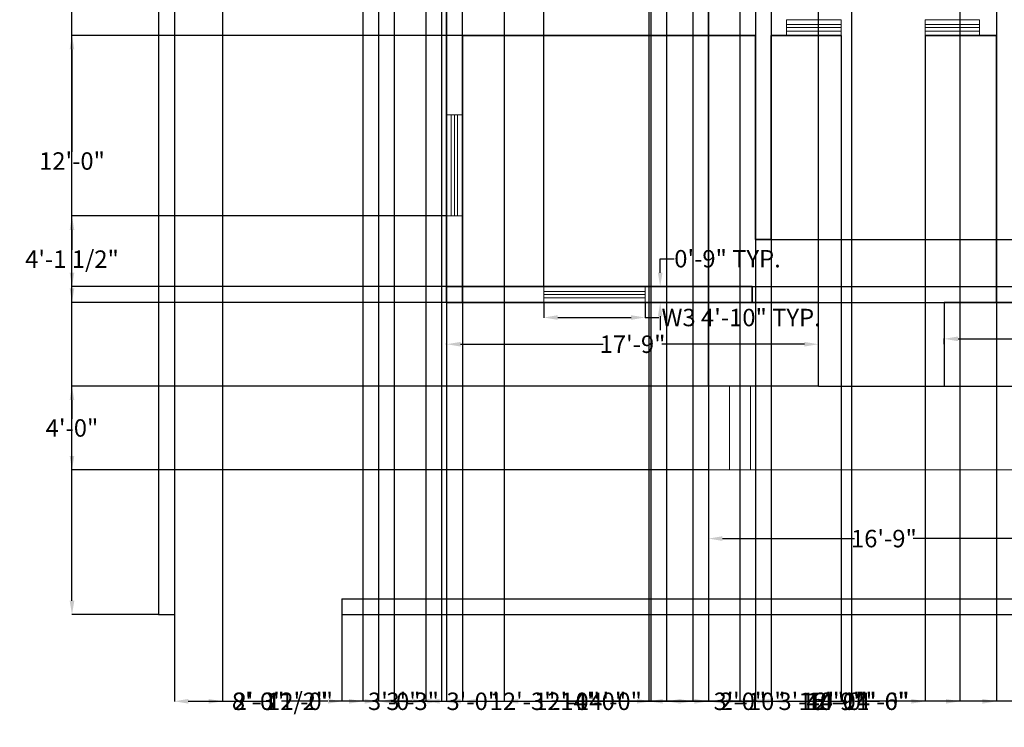
# Model space of a CAD drawing. Units: inches. Extents: x -63 to 800, y 3068 to 4133.
# Tile 1 of 5: x -63 to 501, y 3068 to 3473. Entities that reach past the tile are written whole.
import ezdxf

# ---------------------------------------------------------------- set-up
doc = ezdxf.new("R2010")
doc.units = ezdxf.units.IN
doc.header["$MEASUREMENT"] = 0
for name, color, linetype, lineweight in [('A-ANNO-DIMS', 2, 'Continuous', 13), ('A-FLOR', 7, 'Continuous', 25), ('A-FLOR-STRS', 3, 'Continuous', 18), ('A-GLAZ', 4, 'Continuous', 18), ('A-WALL', 7, 'Continuous', 35), ('A-WALL-SITE', 8, 'Continuous', 30)]:
    doc.layers.add(name, color=color, linetype=linetype, lineweight=lineweight)
doc.styles.get("Standard").update_dxf_attribs({"font": 'arial.ttf'})
doc.dimstyles.get("Standard").update_dxf_attribs({"dimtxt": 10, "dimasz": 8, "dimexe": 0.18, "dimexo": 0.0625, "dimgap": 0.09, "dimtad": 0, "dimtih": 1, "dimtoh": 1, "dimdec": 0, "dimzin": 0, "dimdsep": 46, "dimlunit": 3, "dimtxsty": 'Standard', "dimcen": 0.09, "dimadec": 0, "dimazin": 0, "dimtfac": 1, "dimtdec": 0, "dimtofl": 0, "dimtmove": 0, "dimatfit": 3, "dimfxl": 1, "dimtolj": 1, "dimtzin": 0, "dimarcsym": 0})

# ---------------------------------------------------------------- blocks, each defined once
blk = doc.blocks.new('*D7')
at = {"layer": 'A-ANNO-DIMS', "color": 0, "lineweight": -2, "transparency": 16777216}
for p, q in [((331.31, 3215.25), (331.31, 3175.73)), ((532.31, 3215.25), (532.31, 3175.73)), ((339.31, 3175.91), (415.01, 3175.91)), ((524.31, 3175.91), (448.6, 3175.91))]:
    blk.add_line(p, q, dxfattribs=at)
at = {"layer": 'A-ANNO-DIMS', "color": 0, "transparency": 16777216}
for points in [[(339.31, 3177.24), (339.31, 3174.58), (331.31, 3175.91)], [(524.31, 3177.24), (524.31, 3174.58), (532.31, 3175.91)]]:
    blk.add_solid(points, dxfattribs=at)
at = {"layer": 'Defpoints', "color": 0, "transparency": 16777216}
for p in [(331.31, 3215.31), (532.31, 3215.31), (532.31, 3175.91)]:
    blk.add_point(p, dxfattribs=at)
at = {"layer": 'A-ANNO-DIMS', "color": 0, "transparency": 16777216, "insert": (431.81, 3175.91), "char_height": 10, "attachment_point": 5}
blk.add_mtext('\\A1;16\'-9"', dxfattribs=at)
blk = doc.blocks.new('*D8')
at = {"layer": 'A-ANNO-DIMS', "color": 0, "lineweight": -2, "transparency": 16777216}
for p, q in [((181.31, 3287.37), (181.31, 3287.49)), ((189.31, 3287.31), (271.01, 3287.31)), ((386.31, 3287.31), (304.6, 3287.31)), ((394.31, 3287.37), (394.31, 3287.49))]:
    blk.add_line(p, q, dxfattribs=at)
at = {"layer": 'A-ANNO-DIMS', "color": 0, "transparency": 16777216}
for points in [[(189.31, 3288.64), (189.31, 3285.98), (181.31, 3287.31)], [(386.31, 3288.64), (386.31, 3285.98), (394.31, 3287.31)]]:
    blk.add_solid(points, dxfattribs=at)
at = {"layer": 'Defpoints', "color": 0, "transparency": 16777216}
for p in [(181.31, 3287.31), (394.31, 3287.31), (394.31, 3287.31)]:
    blk.add_point(p, dxfattribs=at)
at = {"layer": 'A-ANNO-DIMS', "color": 0, "transparency": 16777216, "insert": (287.81, 3287.31), "char_height": 10, "attachment_point": 5}
blk.add_mtext('\\A1;17\'-9"', dxfattribs=at)
blk = doc.blocks.new('*D9')
at = {"layer": 'A-ANNO-DIMS', "color": 0, "lineweight": -2, "transparency": 16777216}
for p, q in [((466.31, 3287.37), (466.31, 3290.58)), ((474.31, 3290.4), (560.2, 3290.4)), ((662.31, 3290.4), (576.41, 3290.4)), ((670.31, 3287.37), (670.31, 3290.58))]:
    blk.add_line(p, q, dxfattribs=at)
at = {"layer": 'A-ANNO-DIMS', "color": 0, "transparency": 16777216}
for points in [[(474.31, 3291.73), (474.31, 3289.06), (466.31, 3290.4)], [(662.31, 3291.73), (662.31, 3289.06), (670.31, 3290.4)]]:
    blk.add_solid(points, dxfattribs=at)
at = {"layer": 'Defpoints', "color": 0, "transparency": 16777216}
for p in [(670.31, 3290.4), (466.31, 3287.31), (670.31, 3287.31)]:
    blk.add_point(p, dxfattribs=at)
at = {"layer": 'A-ANNO-DIMS', "color": 0, "transparency": 16777216, "insert": (568.31, 3290.4), "char_height": 10, "attachment_point": 5}
blk.add_mtext("\\A1;17'", dxfattribs=at)
blk = doc.blocks.new('WIN-31')
blk.add_lwpolyline([(0, 9), (31.17, 9), (31.17, 0), (0, 0)], close=True)
blk.add_lwpolyline([(0, 4.5), (31.17, 4.5), (31.17, 6.29), (0, 6.29), (0, 2.51), (31.17, 2.51)])
blk = doc.blocks.new('WIN-58')
blk.add_lwpolyline([(0, 9), (57.99, 9), (57.99, 0), (0, 0)], close=True)
for points in [[(0, 4.5), (57.99, 4.5), (57.99, 6.29), (0, 6.29)], [(0, 2.51), (57.99, 2.51)]]:
    blk.add_lwpolyline(points)
blk = doc.blocks.new('*D17')
at = {"layer": 'A-ANNO-DIMS', "color": 0, "lineweight": -2, "transparency": 16777216}
for p, q in [((236.97, 3311.25), (236.97, 3302.43)), ((294.96, 3311.25), (294.96, 3302.43)), ((244.97, 3302.61), (286.96, 3302.61)), ((294.96, 3302.61), (302.96, 3302.61))]:
    blk.add_line(p, q, dxfattribs=at)
at = {"layer": 'A-ANNO-DIMS', "color": 0, "transparency": 16777216}
for points in [[(244.97, 3303.94), (244.97, 3301.28), (236.97, 3302.61)], [(286.96, 3303.94), (286.96, 3301.28), (294.96, 3302.61)]]:
    blk.add_solid(points, dxfattribs=at)
at = {"layer": 'Defpoints', "color": 0, "transparency": 16777216}
for p in [(236.97, 3311.31), (294.96, 3311.31), (294.96, 3302.61)]:
    blk.add_point(p, dxfattribs=at)
at = {"layer": 'A-ANNO-DIMS', "color": 0, "transparency": 16777216, "insert": (350.04, 3302.61), "char_height": 10, "attachment_point": 5}
blk.add_mtext('\\A1;W3 4\'-10" TYP.', dxfattribs=at)
blk = doc.blocks.new('*D18')
at = {"layer": 'A-ANNO-DIMS', "color": 0, "lineweight": -2, "transparency": 16777216}
for p, q in [((303.66, 3328.31), (303.66, 3336.31)), ((303.66, 3336.31), (311.66, 3336.31)), ((295.02, 3320.31), (303.84, 3320.31)), ((295.02, 3311.31), (303.84, 3311.31)), ((303.66, 3303.31), (303.66, 3295.31))]:
    blk.add_line(p, q, dxfattribs=at)
at = {"layer": 'A-ANNO-DIMS', "color": 0, "transparency": 16777216}
for points in [[(302.33, 3328.31), (304.99, 3328.31), (303.66, 3320.31)], [(302.33, 3303.31), (304.99, 3303.31), (303.66, 3311.31)]]:
    blk.add_solid(points, dxfattribs=at)
at = {"layer": 'Defpoints', "color": 0, "transparency": 16777216}
for p in [(294.96, 3320.31), (303.66, 3320.31), (294.96, 3311.31)]:
    blk.add_point(p, dxfattribs=at)
at = {"layer": 'A-ANNO-DIMS', "color": 0, "transparency": 16777216, "insert": (342.23, 3336.31), "char_height": 10, "attachment_point": 5}
blk.add_mtext('\\A1;0\'-9" TYP.', dxfattribs=at)
blk = doc.blocks.new('*D20')
at = {"layer": 'A-ANNO-DIMS', "color": 0, "lineweight": -2, "transparency": 16777216}
for p, q in [((16.25, 4068.66), (-33.52, 4068.66)), ((-33.34, 4060.66), (-33.34, 3605.75)), ((-33.34, 3140.31), (-33.34, 3595.23)), ((16.25, 3132.31), (-33.52, 3132.31))]:
    blk.add_line(p, q, dxfattribs=at)
at = {"layer": 'A-ANNO-DIMS', "color": 0, "transparency": 16777216}
for points in [[(-34.67, 4060.66), (-32.01, 4060.66), (-33.34, 4068.66)], [(-34.67, 3140.31), (-32.01, 3140.31), (-33.34, 3132.31)]]:
    blk.add_solid(points, dxfattribs=at)
at = {"layer": 'Defpoints', "color": 0, "transparency": 16777216}
for p in [(-33.34, 4068.66), (16.31, 4068.66), (16.31, 3132.31)]:
    blk.add_point(p, dxfattribs=at)
at = {"layer": 'A-ANNO-DIMS', "color": 0, "transparency": 16777216, "insert": (-33.34, 3600.49), "char_height": 10, "attachment_point": 5}
blk.add_mtext('\\A1;78\'-0 1/2"', dxfattribs=at)
blk = doc.blocks.new('*D21')
at = {"layer": 'A-ANNO-DIMS', "color": 0, "lineweight": -2, "transparency": 16777216}
for p, q in [((25.31, 3132.25), (25.31, 3082.48)), ((121.31, 3132.25), (121.31, 3082.48)), ((33.31, 3082.66), (59.92, 3082.66)), ((113.31, 3082.66), (86.7, 3082.66))]:
    blk.add_line(p, q, dxfattribs=at)
at = {"layer": 'A-ANNO-DIMS', "color": 0, "transparency": 16777216}
for points in [[(33.31, 3083.99), (33.31, 3081.33), (25.31, 3082.66)], [(113.31, 3083.99), (113.31, 3081.33), (121.31, 3082.66)]]:
    blk.add_solid(points, dxfattribs=at)
at = {"layer": 'Defpoints', "color": 0, "transparency": 16777216}
for p in [(25.31, 3132.31), (121.31, 3132.31), (121.31, 3082.66)]:
    blk.add_point(p, dxfattribs=at)
at = {"layer": 'A-ANNO-DIMS', "color": 0, "transparency": 16777216, "insert": (73.31, 3082.66), "char_height": 10, "attachment_point": 5}
blk.add_mtext('\\A1;8\'-0"', dxfattribs=at)
blk = doc.blocks.new('*D23')
at = {"layer": 'A-ANNO-DIMS', "color": 0, "lineweight": -2, "transparency": 16777216}
for p, q in [((25.31, 4059.6), (25.31, 3082.48)), ((169.31, 4059.6), (169.31, 3082.48)), ((33.31, 3082.66), (80.51, 3082.66)), ((161.31, 3082.66), (114.1, 3082.66))]:
    blk.add_line(p, q, dxfattribs=at)
at = {"layer": 'A-ANNO-DIMS', "color": 0, "transparency": 16777216}
for points in [[(33.31, 3083.99), (33.31, 3081.33), (25.31, 3082.66)], [(161.31, 3083.99), (161.31, 3081.33), (169.31, 3082.66)]]:
    blk.add_solid(points, dxfattribs=at)
at = {"layer": 'Defpoints', "color": 0, "transparency": 16777216}
for p in [(25.31, 4059.66), (169.31, 4059.66), (169.31, 3082.66)]:
    blk.add_point(p, dxfattribs=at)
at = {"layer": 'A-ANNO-DIMS', "color": 0, "transparency": 16777216, "insert": (97.31, 3082.66), "char_height": 10, "attachment_point": 5}
blk.add_mtext('\\A1;12\'-0"', dxfattribs=at)
blk = doc.blocks.new('*D24')
at = {"layer": 'A-ANNO-DIMS', "color": 0, "lineweight": -2, "transparency": 16777216}
for p, q in [((178.31, 4059.6), (178.31, 3082.48)), ((322.31, 4059.6), (322.31, 3082.48)), ((186.31, 3082.66), (233.51, 3082.66)), ((314.31, 3082.66), (267.1, 3082.66))]:
    blk.add_line(p, q, dxfattribs=at)
at = {"layer": 'A-ANNO-DIMS', "color": 0, "transparency": 16777216}
for points in [[(186.31, 3083.99), (186.31, 3081.33), (178.31, 3082.66)], [(314.31, 3083.99), (314.31, 3081.33), (322.31, 3082.66)]]:
    blk.add_solid(points, dxfattribs=at)
at = {"layer": 'Defpoints', "color": 0, "transparency": 16777216}
for p in [(178.31, 4059.66), (322.31, 4059.66), (322.31, 3082.66)]:
    blk.add_point(p, dxfattribs=at)
at = {"layer": 'A-ANNO-DIMS', "color": 0, "transparency": 16777216, "insert": (250.31, 3082.66), "char_height": 10, "attachment_point": 5}
blk.add_mtext('\\A1;12\'-0"', dxfattribs=at)
blk = doc.blocks.new('*D25')
at = {"layer": 'A-ANNO-DIMS', "color": 0, "lineweight": -2, "transparency": 16777216}
for p, q in [((331.31, 4059.6), (331.31, 3082.48)), ((475.31, 4059.6), (475.31, 3082.48)), ((339.31, 3082.66), (386.51, 3082.66)), ((467.31, 3082.66), (420.1, 3082.66))]:
    blk.add_line(p, q, dxfattribs=at)
at = {"layer": 'A-ANNO-DIMS', "color": 0, "transparency": 16777216}
for points in [[(339.31, 3083.99), (339.31, 3081.33), (331.31, 3082.66)], [(467.31, 3083.99), (467.31, 3081.33), (475.31, 3082.66)]]:
    blk.add_solid(points, dxfattribs=at)
at = {"layer": 'Defpoints', "color": 0, "transparency": 16777216}
for p in [(331.31, 4059.66), (475.31, 4059.66), (475.31, 3082.66)]:
    blk.add_point(p, dxfattribs=at)
at = {"layer": 'A-ANNO-DIMS', "color": 0, "transparency": 16777216, "insert": (403.31, 3082.66), "char_height": 10, "attachment_point": 5}
blk.add_mtext('\\A1;12\'-0"', dxfattribs=at)
blk = doc.blocks.new('*D27')
at = {"layer": 'A-ANNO-DIMS', "color": 0, "lineweight": -2, "transparency": 16777216}
for p, q in [((25.31, 3951.6), (25.31, 3082.48)), ((52.97, 3951.6), (52.97, 3082.48)), ((33.31, 3082.66), (44.97, 3082.66)), ((52.97, 3082.66), (60.97, 3082.66))]:
    blk.add_line(p, q, dxfattribs=at)
at = {"layer": 'A-ANNO-DIMS', "color": 0, "transparency": 16777216}
for points in [[(33.31, 3083.99), (33.31, 3081.33), (25.31, 3082.66)], [(44.97, 3083.99), (44.97, 3081.33), (52.97, 3082.66)]]:
    blk.add_solid(points, dxfattribs=at)
at = {"layer": 'Defpoints', "color": 0, "transparency": 16777216}
for p in [(25.31, 3951.66), (52.97, 3951.66), (52.97, 3082.66)]:
    blk.add_point(p, dxfattribs=at)
at = {"layer": 'A-ANNO-DIMS', "color": 0, "transparency": 16777216, "insert": (86.08, 3082.66), "char_height": 10, "attachment_point": 5}
blk.add_mtext('\\A1;2\'-3 1/2"', dxfattribs=at)
blk = doc.blocks.new('*D28')
at = {"layer": 'A-ANNO-DIMS', "color": 0, "lineweight": -2, "transparency": 16777216}
for p, q in [((297.16, 3951.55), (297.16, 3082.48)), ((331.31, 3951.6), (331.31, 3082.48)), ((305.16, 3082.66), (323.31, 3082.66)), ((331.31, 3082.66), (339.31, 3082.66))]:
    blk.add_line(p, q, dxfattribs=at)
at = {"layer": 'A-ANNO-DIMS', "color": 0, "transparency": 16777216}
for points in [[(305.16, 3083.99), (305.16, 3081.33), (297.16, 3082.66)], [(323.31, 3083.99), (323.31, 3081.33), (331.31, 3082.66)]]:
    blk.add_solid(points, dxfattribs=at)
at = {"layer": 'Defpoints', "color": 0, "transparency": 16777216}
for p in [(297.16, 3951.61), (331.31, 3951.66), (331.31, 3082.66)]:
    blk.add_point(p, dxfattribs=at)
at = {"layer": 'A-ANNO-DIMS', "color": 0, "transparency": 16777216, "insert": (356.66, 3082.66), "char_height": 10, "attachment_point": 5}
blk.add_mtext('\\A1;2\'-10"', dxfattribs=at)
blk = doc.blocks.new('*D29')
at = {"layer": 'A-ANNO-DIMS', "color": 0, "lineweight": -2, "transparency": 16777216}
for p, q in [((367.31, 3951.6), (367.31, 3082.48)), ((413.21, 3951.6), (413.21, 3082.48)), ((359.31, 3082.66), (351.31, 3082.66)), ((421.21, 3082.66), (429.21, 3082.66))]:
    blk.add_line(p, q, dxfattribs=at)
at = {"layer": 'A-ANNO-DIMS', "color": 0, "transparency": 16777216}
for points in [[(359.31, 3083.99), (359.31, 3081.33), (367.31, 3082.66)], [(421.21, 3083.99), (421.21, 3081.33), (413.21, 3082.66)]]:
    blk.add_solid(points, dxfattribs=at)
at = {"layer": 'Defpoints', "color": 0, "transparency": 16777216}
for p in [(367.31, 3951.66), (413.21, 3951.66), (413.21, 3082.66)]:
    blk.add_point(p, dxfattribs=at)
at = {"layer": 'A-ANNO-DIMS', "color": 0, "transparency": 16777216, "insert": (390.26, 3082.66), "char_height": 10, "attachment_point": 5}
blk.add_mtext('\\A1;3\'-10"', dxfattribs=at)
blk = doc.blocks.new('*D30')
at = {"layer": 'A-ANNO-DIMS', "color": 0, "lineweight": -2, "transparency": 16777216}
for p, q in [((133.31, 3951.6), (133.31, 3082.48)), ((169.31, 3951.6), (169.31, 3082.48)), ((125.31, 3082.66), (117.31, 3082.66)), ((177.31, 3082.66), (185.31, 3082.66))]:
    blk.add_line(p, q, dxfattribs=at)
at = {"layer": 'A-ANNO-DIMS', "color": 0, "transparency": 16777216}
for points in [[(125.31, 3083.99), (125.31, 3081.33), (133.31, 3082.66)], [(177.31, 3083.99), (177.31, 3081.33), (169.31, 3082.66)]]:
    blk.add_solid(points, dxfattribs=at)
at = {"layer": 'Defpoints', "color": 0, "transparency": 16777216}
for p in [(133.31, 3951.66), (169.31, 3951.66), (169.31, 3082.66)]:
    blk.add_point(p, dxfattribs=at)
at = {"layer": 'A-ANNO-DIMS', "color": 0, "transparency": 16777216, "insert": (151.31, 3082.66), "char_height": 10, "attachment_point": 5}
blk.add_mtext('\\A1;3\'-0"', dxfattribs=at)
blk = doc.blocks.new('*D31')
at = {"layer": 'A-ANNO-DIMS', "color": 0, "lineweight": -2, "transparency": 16777216}
for p, q in [((178.31, 3951.6), (178.31, 3082.48)), ((214.31, 3951.6), (214.31, 3082.48)), ((170.31, 3082.66), (162.31, 3082.66)), ((222.31, 3082.66), (230.31, 3082.66))]:
    blk.add_line(p, q, dxfattribs=at)
at = {"layer": 'A-ANNO-DIMS', "color": 0, "transparency": 16777216}
for points in [[(170.31, 3083.99), (170.31, 3081.33), (178.31, 3082.66)], [(222.31, 3083.99), (222.31, 3081.33), (214.31, 3082.66)]]:
    blk.add_solid(points, dxfattribs=at)
at = {"layer": 'Defpoints', "color": 0, "transparency": 16777216}
for p in [(178.31, 3951.66), (214.31, 3951.66), (214.31, 3082.66)]:
    blk.add_point(p, dxfattribs=at)
at = {"layer": 'A-ANNO-DIMS', "color": 0, "transparency": 16777216, "insert": (196.31, 3082.66), "char_height": 10, "attachment_point": 5}
blk.add_mtext('\\A1;3\'-0"', dxfattribs=at)
blk = doc.blocks.new('*D32')
at = {"layer": 'A-ANNO-DIMS', "color": 0, "lineweight": -2, "transparency": 16777216}
for p, q in [((331.31, 3951.6), (331.31, 3082.48)), ((367.31, 3951.6), (367.31, 3082.48)), ((323.31, 3082.66), (315.31, 3082.66)), ((375.31, 3082.66), (383.31, 3082.66))]:
    blk.add_line(p, q, dxfattribs=at)
at = {"layer": 'A-ANNO-DIMS', "color": 0, "transparency": 16777216}
for points in [[(323.31, 3083.99), (323.31, 3081.33), (331.31, 3082.66)], [(375.31, 3083.99), (375.31, 3081.33), (367.31, 3082.66)]]:
    blk.add_solid(points, dxfattribs=at)
at = {"layer": 'Defpoints', "color": 0, "transparency": 16777216}
for p in [(331.31, 3951.66), (367.31, 3951.66), (367.31, 3082.66)]:
    blk.add_point(p, dxfattribs=at)
at = {"layer": 'A-ANNO-DIMS', "color": 0, "transparency": 16777216, "insert": (349.31, 3082.66), "char_height": 10, "attachment_point": 5}
blk.add_mtext('\\A1;3\'-0"', dxfattribs=at)
blk = doc.blocks.new('*D34')
at = {"layer": 'A-ANNO-DIMS', "color": 0, "lineweight": -2, "transparency": 16777216}
for p, q in [((142.31, 3522.75), (142.31, 3082.48)), ((670.31, 3263.25), (670.31, 3082.48)), ((150.31, 3082.66), (388.84, 3082.66)), ((662.31, 3082.66), (423.78, 3082.66))]:
    blk.add_line(p, q, dxfattribs=at)
at = {"layer": 'A-ANNO-DIMS', "color": 0, "transparency": 16777216}
for points in [[(150.31, 3083.99), (150.31, 3081.33), (142.31, 3082.66)], [(662.31, 3083.99), (662.31, 3081.33), (670.31, 3082.66)]]:
    blk.add_solid(points, dxfattribs=at)
at = {"layer": 'Defpoints', "color": 0, "transparency": 16777216}
for p in [(142.31, 3522.81), (670.31, 3263.31), (670.31, 3082.66)]:
    blk.add_point(p, dxfattribs=at)
at = {"layer": 'A-ANNO-DIMS', "color": 0, "transparency": 16777216, "insert": (406.31, 3082.66), "char_height": 10, "attachment_point": 5}
blk.add_mtext('\\A1;44\'-0"', dxfattribs=at)
blk = doc.blocks.new('*D37')
at = {"layer": 'A-ANNO-DIMS', "color": 0, "lineweight": -2, "transparency": 16777216}
for p, q in [((181.31, 3885.75), (181.31, 3082.48)), ((349.31, 3885.75), (349.31, 3082.48)), ((189.31, 3082.66), (248.51, 3082.66)), ((341.31, 3082.66), (282.1, 3082.66))]:
    blk.add_line(p, q, dxfattribs=at)
at = {"layer": 'A-ANNO-DIMS', "color": 0, "transparency": 16777216}
for points in [[(189.31, 3083.99), (189.31, 3081.33), (181.31, 3082.66)], [(341.31, 3083.99), (341.31, 3081.33), (349.31, 3082.66)]]:
    blk.add_solid(points, dxfattribs=at)
at = {"layer": 'Defpoints', "color": 0, "transparency": 16777216}
for p in [(181.31, 3885.81), (349.31, 3885.81), (349.31, 3082.66)]:
    blk.add_point(p, dxfattribs=at)
at = {"layer": 'A-ANNO-DIMS', "color": 0, "transparency": 16777216, "insert": (265.31, 3082.66), "char_height": 10, "attachment_point": 5}
blk.add_mtext('\\A1;14\'-0"', dxfattribs=at)
blk = doc.blocks.new('*D38')
at = {"layer": 'A-ANNO-DIMS', "color": 0, "lineweight": -2, "transparency": 16777216}
for p, q in [((358.31, 3885.75), (358.31, 3082.48)), ((496.31, 3885.75), (496.31, 3082.48)), ((366.31, 3082.66), (410.51, 3082.66)), ((488.31, 3082.66), (444.1, 3082.66))]:
    blk.add_line(p, q, dxfattribs=at)
at = {"layer": 'A-ANNO-DIMS', "color": 0, "transparency": 16777216}
for points in [[(366.31, 3083.99), (366.31, 3081.33), (358.31, 3082.66)], [(488.31, 3083.99), (488.31, 3081.33), (496.31, 3082.66)]]:
    blk.add_solid(points, dxfattribs=at)
at = {"layer": 'Defpoints', "color": 0, "transparency": 16777216}
for p in [(358.31, 3885.81), (496.31, 3885.81), (496.31, 3082.66)]:
    blk.add_point(p, dxfattribs=at)
at = {"layer": 'A-ANNO-DIMS', "color": 0, "transparency": 16777216, "insert": (427.31, 3082.66), "char_height": 10, "attachment_point": 5}
blk.add_mtext('\\A1;11\'-6"', dxfattribs=at)
blk = doc.blocks.new('*D44')
at = {"layer": 'A-ANNO-DIMS', "color": 0, "lineweight": -2, "transparency": 16777216}
for p, q in [((151.31, 3732.75), (151.31, 3082.48)), ((298.31, 3732.75), (298.31, 3082.48)), ((159.31, 3082.66), (208.01, 3082.66)), ((290.31, 3082.66), (241.6, 3082.66))]:
    blk.add_line(p, q, dxfattribs=at)
at = {"layer": 'A-ANNO-DIMS', "color": 0, "transparency": 16777216}
for points in [[(159.31, 3083.99), (159.31, 3081.33), (151.31, 3082.66)], [(290.31, 3083.99), (290.31, 3081.33), (298.31, 3082.66)]]:
    blk.add_solid(points, dxfattribs=at)
at = {"layer": 'Defpoints', "color": 0, "transparency": 16777216}
for p in [(151.31, 3732.81), (298.31, 3732.81), (298.31, 3082.66)]:
    blk.add_point(p, dxfattribs=at)
at = {"layer": 'A-ANNO-DIMS', "color": 0, "transparency": 16777216, "insert": (224.81, 3082.66), "char_height": 10, "attachment_point": 5}
blk.add_mtext('\\A1;12\'-3"', dxfattribs=at)
blk = doc.blocks.new('*D45')
at = {"layer": 'A-ANNO-DIMS', "color": 0, "lineweight": -2, "transparency": 16777216}
for p, q in [((307.31, 3732.75), (307.31, 3082.48)), ((496.31, 3732.75), (496.31, 3082.48)), ((315.31, 3082.66), (385.01, 3082.66)), ((488.31, 3082.66), (418.6, 3082.66))]:
    blk.add_line(p, q, dxfattribs=at)
at = {"layer": 'A-ANNO-DIMS', "color": 0, "transparency": 16777216}
for points in [[(315.31, 3083.99), (315.31, 3081.33), (307.31, 3082.66)], [(488.31, 3083.99), (488.31, 3081.33), (496.31, 3082.66)]]:
    blk.add_solid(points, dxfattribs=at)
at = {"layer": 'Defpoints', "color": 0, "transparency": 16777216}
for p in [(307.31, 3732.81), (496.31, 3732.81), (496.31, 3082.66)]:
    blk.add_point(p, dxfattribs=at)
at = {"layer": 'A-ANNO-DIMS', "color": 0, "transparency": 16777216, "insert": (401.81, 3082.66), "char_height": 10, "attachment_point": 5}
blk.add_mtext('\\A1;15\'-9"', dxfattribs=at)
blk = doc.blocks.new('*D51')
at = {"layer": 'A-ANNO-DIMS', "color": 0, "lineweight": -2, "transparency": 16777216}
for p, q in [((190.31, 3464.25), (190.31, 3082.48)), ((358.31, 3464.25), (358.31, 3082.48)), ((198.31, 3082.66), (257.51, 3082.66)), ((350.31, 3082.66), (291.1, 3082.66))]:
    blk.add_line(p, q, dxfattribs=at)
at = {"layer": 'A-ANNO-DIMS', "color": 0, "transparency": 16777216}
for points in [[(198.31, 3083.99), (198.31, 3081.33), (190.31, 3082.66)], [(350.31, 3083.99), (350.31, 3081.33), (358.31, 3082.66)]]:
    blk.add_solid(points, dxfattribs=at)
at = {"layer": 'Defpoints', "color": 0, "transparency": 16777216}
for p in [(190.31, 3464.31), (358.31, 3464.31), (358.31, 3082.66)]:
    blk.add_point(p, dxfattribs=at)
at = {"layer": 'A-ANNO-DIMS', "color": 0, "transparency": 16777216, "insert": (274.31, 3082.66), "char_height": 10, "attachment_point": 5}
blk.add_mtext('\\A1;14\'-0"', dxfattribs=at)
blk = doc.blocks.new('*D52')
at = {"layer": 'A-ANNO-DIMS', "color": 0, "lineweight": -2, "transparency": 16777216}
for p, q in [((358.25, 3464.31), (-33.52, 3464.31)), ((-33.34, 3456.31), (-33.34, 3397.51)), ((-33.34, 3328.31), (-33.34, 3387.11)), ((356.25, 3320.31), (-33.52, 3320.31))]:
    blk.add_line(p, q, dxfattribs=at)
at = {"layer": 'A-ANNO-DIMS', "color": 0, "transparency": 16777216}
for points in [[(-34.67, 3456.31), (-32.01, 3456.31), (-33.34, 3464.31)], [(-34.67, 3328.31), (-32.01, 3328.31), (-33.34, 3320.31)]]:
    blk.add_solid(points, dxfattribs=at)
at = {"layer": 'Defpoints', "color": 0, "transparency": 16777216}
for p in [(-33.34, 3464.31), (358.31, 3464.31), (356.31, 3320.31)]:
    blk.add_point(p, dxfattribs=at)
at = {"layer": 'A-ANNO-DIMS', "color": 0, "transparency": 16777216, "insert": (-33.34, 3392.31), "char_height": 10, "attachment_point": 5}
blk.add_mtext('\\A1;12\'-0"', dxfattribs=at)
blk = doc.blocks.new('*D55')
at = {"layer": 'A-ANNO-DIMS', "color": 0, "lineweight": -2, "transparency": 16777216}
for p, q in [((394.37, 3311.31), (771.14, 3311.31)), ((770.96, 3303.31), (770.96, 3292.51)), ((770.96, 3271.31), (770.96, 3282.11)), ((394.37, 3263.31), (771.14, 3263.31))]:
    blk.add_line(p, q, dxfattribs=at)
at = {"layer": 'A-ANNO-DIMS', "color": 0, "transparency": 16777216}
for points in [[(769.63, 3303.31), (772.29, 3303.31), (770.96, 3311.31)], [(769.63, 3271.31), (772.29, 3271.31), (770.96, 3263.31)]]:
    blk.add_solid(points, dxfattribs=at)
at = {"layer": 'Defpoints', "color": 0, "transparency": 16777216}
for p in [(394.31, 3311.31), (770.96, 3311.31), (394.31, 3263.31)]:
    blk.add_point(p, dxfattribs=at)
at = {"layer": 'A-ANNO-DIMS', "color": 0, "transparency": 16777216, "insert": (770.96, 3287.31), "char_height": 10, "attachment_point": 5}
blk.add_mtext('\\A1;4\'-0"', dxfattribs=at)
blk = doc.blocks.new('*D56')
at = {"layer": 'A-ANNO-DIMS', "color": 0, "lineweight": -2, "transparency": 16777216}
for p, q in [((331.25, 3263.31), (-33.52, 3263.31)), ((-33.34, 3255.31), (-33.34, 3244.51)), ((-33.34, 3223.31), (-33.34, 3234.11)), ((331.25, 3215.31), (-33.52, 3215.31))]:
    blk.add_line(p, q, dxfattribs=at)
at = {"layer": 'A-ANNO-DIMS', "color": 0, "transparency": 16777216}
for points in [[(-34.67, 3255.31), (-32.01, 3255.31), (-33.34, 3263.31)], [(-34.67, 3223.31), (-32.01, 3223.31), (-33.34, 3215.31)]]:
    blk.add_solid(points, dxfattribs=at)
at = {"layer": 'Defpoints', "color": 0, "transparency": 16777216}
for p in [(-33.34, 3263.31), (331.31, 3263.31), (331.31, 3215.31)]:
    blk.add_point(p, dxfattribs=at)
at = {"layer": 'A-ANNO-DIMS', "color": 0, "transparency": 16777216, "insert": (-33.34, 3239.31), "char_height": 10, "attachment_point": 5}
blk.add_mtext('\\A1;4\'-0"', dxfattribs=at)
blk = doc.blocks.new('*D57')
at = {"layer": 'A-ANNO-DIMS', "color": 0, "lineweight": -2, "transparency": 16777216}
for p, q in [((190.31, 3311.37), (190.31, 4118.49)), ((198.31, 4118.31), (228.97, 4118.31)), ((236.97, 3320.37), (236.97, 4118.49)), ((236.97, 4118.31), (244.97, 4118.31))]:
    blk.add_line(p, q, dxfattribs=at)
at = {"layer": 'A-ANNO-DIMS', "color": 0, "transparency": 16777216}
for points in [[(198.31, 4119.64), (198.31, 4116.98), (190.31, 4118.31)], [(228.97, 4119.64), (228.97, 4116.98), (236.97, 4118.31)]]:
    blk.add_solid(points, dxfattribs=at)
at = {"layer": 'Defpoints', "color": 0, "transparency": 16777216}
for p in [(236.97, 4118.31), (236.97, 3320.31), (190.31, 3311.31)]:
    blk.add_point(p, dxfattribs=at)
at = {"layer": 'A-ANNO-DIMS', "color": 0, "transparency": 16777216, "insert": (273.88, 4118.31), "char_height": 10, "attachment_point": 5}
blk.add_mtext('\\A1;3\'-10 1/2"', dxfattribs=at)
blk = doc.blocks.new('*D59')
at = {"layer": 'A-ANNO-DIMS', "color": 0, "lineweight": -2, "transparency": 16777216}
for p, q in [((181.25, 3360.81), (-33.52, 3360.81)), ((-33.34, 3352.81), (-33.34, 3341.32)), ((-33.34, 3319.31), (-33.34, 3330.8)), ((181.25, 3311.31), (-33.52, 3311.31))]:
    blk.add_line(p, q, dxfattribs=at)
at = {"layer": 'A-ANNO-DIMS', "color": 0, "transparency": 16777216}
for points in [[(-34.67, 3352.81), (-32.01, 3352.81), (-33.34, 3360.81)], [(-34.67, 3319.31), (-32.01, 3319.31), (-33.34, 3311.31)]]:
    blk.add_solid(points, dxfattribs=at)
at = {"layer": 'Defpoints', "color": 0, "transparency": 16777216}
for p in [(-33.34, 3360.81), (181.31, 3360.81), (181.31, 3311.31)]:
    blk.add_point(p, dxfattribs=at)
at = {"layer": 'A-ANNO-DIMS', "color": 0, "transparency": 16777216, "insert": (-33.34, 3336.06), "char_height": 10, "attachment_point": 5}
blk.add_mtext('\\A1;4\'-1 1/2"', dxfattribs=at)
blk = doc.blocks.new('*D61')
at = {"layer": 'A-ANNO-DIMS', "color": 0, "lineweight": -2, "transparency": 16777216}
for p, q in [((407.28, 3464.25), (407.28, 3082.48)), ((455.48, 3464.25), (455.48, 3082.48)), ((415.28, 3082.66), (417.8, 3082.66)), ((447.48, 3082.66), (444.96, 3082.66))]:
    blk.add_line(p, q, dxfattribs=at)
at = {"layer": 'A-ANNO-DIMS', "color": 0, "transparency": 16777216}
for points in [[(415.28, 3083.99), (415.28, 3081.33), (407.28, 3082.66)], [(447.48, 3083.99), (447.48, 3081.33), (455.48, 3082.66)]]:
    blk.add_solid(points, dxfattribs=at)
at = {"layer": 'Defpoints', "color": 0, "transparency": 16777216}
for p in [(407.28, 3464.31), (455.48, 3464.31), (455.48, 3082.66)]:
    blk.add_point(p, dxfattribs=at)
at = {"layer": 'A-ANNO-DIMS', "color": 0, "transparency": 16777216, "insert": (431.38, 3082.66), "char_height": 10, "attachment_point": 5}
blk.add_mtext('\\A1;4\'-0"', dxfattribs=at)
blk = doc.blocks.new('*D69')
at = {"layer": 'A-ANNO-DIMS', "color": 0, "lineweight": -2, "transparency": 16777216}
for p, q in [((142.31, 3522.75), (142.31, 3082.48)), ((181.31, 3522.75), (181.31, 3082.48)), ((134.31, 3082.66), (126.31, 3082.66)), ((189.31, 3082.66), (197.31, 3082.66))]:
    blk.add_line(p, q, dxfattribs=at)
at = {"layer": 'A-ANNO-DIMS', "color": 0, "transparency": 16777216}
for points in [[(134.31, 3083.99), (134.31, 3081.33), (142.31, 3082.66)], [(189.31, 3083.99), (189.31, 3081.33), (181.31, 3082.66)]]:
    blk.add_solid(points, dxfattribs=at)
at = {"layer": 'Defpoints', "color": 0, "transparency": 16777216}
for p in [(142.31, 3522.81), (181.31, 3522.81), (181.31, 3082.66)]:
    blk.add_point(p, dxfattribs=at)
at = {"layer": 'A-ANNO-DIMS', "color": 0, "transparency": 16777216, "insert": (161.81, 3082.66), "char_height": 10, "attachment_point": 5}
blk.add_mtext('\\A1;3\'-3"', dxfattribs=at)
blk = doc.blocks.new('*D70')
at = {"layer": 'A-ANNO-DIMS', "color": 0, "lineweight": -2, "transparency": 16777216}
for p, q in [((331.31, 3263.37), (331.31, 4118.49)), ((339.31, 4118.31), (349.43, 4118.31)), ((386.31, 4118.31), (376.19, 4118.31)), ((394.31, 3263.37), (394.31, 4118.49))]:
    blk.add_line(p, q, dxfattribs=at)
at = {"layer": 'A-ANNO-DIMS', "color": 0, "transparency": 16777216}
for points in [[(339.31, 4119.64), (339.31, 4116.98), (331.31, 4118.31)], [(386.31, 4119.64), (386.31, 4116.98), (394.31, 4118.31)]]:
    blk.add_solid(points, dxfattribs=at)
at = {"layer": 'Defpoints', "color": 0, "transparency": 16777216}
for p in [(394.31, 4118.31), (331.31, 3263.31), (394.31, 3263.31)]:
    blk.add_point(p, dxfattribs=at)
at = {"layer": 'A-ANNO-DIMS', "color": 0, "transparency": 16777216, "insert": (362.81, 4118.31), "char_height": 10, "attachment_point": 5}
blk.add_mtext('\\A1;5\'-3"', dxfattribs=at)
blk = doc.blocks.new('*D71')
at = {"layer": 'A-ANNO-DIMS', "color": 0, "lineweight": -2, "transparency": 16777216}
for p, q in [((358.37, 3347.31), (771.14, 3347.31)), ((770.96, 3339.31), (770.96, 3339.01)), ((770.96, 3328.31), (770.96, 3328.61)), ((356.37, 3320.31), (771.14, 3320.31))]:
    blk.add_line(p, q, dxfattribs=at)
at = {"layer": 'A-ANNO-DIMS', "color": 0, "transparency": 16777216}
for points in [[(769.63, 3339.31), (772.29, 3339.31), (770.96, 3347.31)], [(769.63, 3328.31), (772.29, 3328.31), (770.96, 3320.31)]]:
    blk.add_solid(points, dxfattribs=at)
at = {"layer": 'Defpoints', "color": 0, "transparency": 16777216}
for p in [(358.31, 3347.31), (356.31, 3320.31), (770.96, 3320.31)]:
    blk.add_point(p, dxfattribs=at)
at = {"layer": 'A-ANNO-DIMS', "color": 0, "transparency": 16777216, "insert": (770.96, 3333.81), "char_height": 10, "attachment_point": 5}
blk.add_mtext('\\A1;2\'-3"', dxfattribs=at)

msp = doc.modelspace()

# ---------------------------------------------------------------- linework, layer by layer
at = {"layer": 'A-FLOR'}
for p, q in [((181.31, 3311.31), (181.31, 3263.31)), ((367.31, 3311.31), (394.31, 3311.31)), ((394.31, 3263.31), (394.31, 3311.31)), ((466.31, 3311.31), (466.31, 3263.31)), ((466.31, 3311.31), (496.31, 3311.31)), ((394.31, 3263.31), (181.31, 3263.31)), ((466.31, 3263.31), (670.31, 3263.31))]:
    msp.add_line(p, q, dxfattribs=at)
at = {"layer": 'A-FLOR-STRS'}
for p, q in [((331.31, 3263.31), (331.31, 3215.31)), ((343.31, 3263.31), (343.31, 3215.31)), ((355.31, 3263.31), (355.31, 3215.31)), ((355.31, 3263.31), (355.31, 3215.31)), ((367.31, 3263.31), (367.31, 3215.31)), ((496.31, 3263.31), (496.31, 3215.31)), ((367.31, 3215.31), (331.31, 3215.31)), ((331.31, 3215.31), (532.31, 3215.31))]:
    msp.add_line(p, q, dxfattribs=at)
at = {"layer": 'A-WALL'}
for p, q in [((181.31, 3549.81), (181.31, 3311.31)), ((298.31, 3464.31), (190.31, 3464.31)), ((190.31, 3464.31), (190.31, 3311.31)), ((298.31, 3464.31), (358.31, 3464.31)), ((358.31, 3464.31), (358.31, 3347.31)), ((367.31, 3464.31), (367.31, 3347.31)), ((367.31, 3464.31), (407.28, 3464.31)), ((367.31, 3464.31), (407.28, 3464.31)), ((455.48, 3464.31), (496.31, 3464.31)), ((455.48, 3464.31), (496.31, 3464.31)), ((496.31, 3464.31), (496.31, 3311.31)), ((356.31, 3320.31), (181.31, 3320.31)), ((298.31, 3320.31), (356.31, 3320.31)), ((367.31, 3311.31), (181.31, 3311.31)), ((298.31, 3311.31), (394.31, 3311.31)), ((466.31, 3311.31), (670.31, 3311.31))]:
    msp.add_line(p, q, dxfattribs=at)
for points in [[(358.31, 3347.31), (367.31, 3347.31)], [(367.31, 3311.31), (356.31, 3311.31), (356.31, 3320.31)]]:
    msp.add_lwpolyline(points, dxfattribs=at)
at = {"layer": 'A-WALL-SITE'}
for p, q in [((16.31, 4068.66), (16.31, 3132.31)), ((25.31, 3951.66), (25.31, 3132.31)), ((121.31, 3141.31), (616.31, 3141.31)), ((16.31, 3132.31), (25.31, 3132.31)), ((121.31, 3132.31), (616.31, 3132.31))]:
    msp.add_line(p, q, dxfattribs=at)
msp.add_lwpolyline([(121.31, 3141.31), (121.31, 3132.31)], dxfattribs=at)

# ---------------------------------------------------------------- block references
at = {"layer": 'A-GLAZ'}
for name, p in [('WIN-31', (376.11, 3464.31)), ('WIN-31', (455.48, 3464.31)), ('WIN-58', (236.97, 3311.31))]:
    msp.add_blockref(name, p, dxfattribs=at)
at = {"layer": 'A-GLAZ', "rotation": 269.9999999999996}
msp.add_blockref('WIN-58', (181.31, 3418.8), dxfattribs=at)

# ---------------------------------------------------------------- dimensions: what is measured, and where the dimension line sits
at = {"layer": 'A-ANNO-DIMS'}
for base, p1, p2, override, picture, middle in [((236.97, 4118.31), (190.31, 3311.31), (236.97, 3320.31), {"dimdec": 1, "dimlfac": 1, "dimrnd": 0, "dimzin": 1, "dimdsep": 46, "dimlunit": 4, "dimfrac": 2}, '*D57', (273.88, 4118.31)), ((394.31, 4118.31), (331.31, 3263.31), (394.31, 3263.31), {"dimdec": 1, "dimlfac": 1, "dimrnd": 0, "dimzin": 1, "dimdsep": 46, "dimlunit": 4, "dimfrac": 2}, '*D70', (362.81, 4118.31)), ((169.31, 3082.66), (25.31, 4059.66), (169.31, 4059.66), {"dimdec": 1, "dimlfac": 1, "dimrnd": 0, "dimzin": 1, "dimdsep": 46, "dimlunit": 4, "dimfrac": 2}, '*D23', (97.31, 3082.66)), ((322.31, 3082.66), (178.31, 4059.66), (322.31, 4059.66), {"dimdec": 1, "dimlfac": 1, "dimrnd": 0, "dimzin": 1, "dimdsep": 46, "dimlunit": 4, "dimfrac": 2}, '*D24', (250.31, 3082.66)), ((475.31, 3082.66), (331.31, 4059.66), (475.31, 4059.66), {"dimdec": 1, "dimlfac": 1, "dimrnd": 0, "dimzin": 1, "dimdsep": 46, "dimlunit": 4, "dimfrac": 2}, '*D25', (403.31, 3082.66)), ((52.97, 3082.66), (25.31, 3951.66), (52.97, 3951.66), {"dimdec": 1, "dimlfac": 1, "dimrnd": 0, "dimzin": 1, "dimdsep": 46, "dimlunit": 4, "dimfrac": 2}, '*D27', (86.08, 3082.66)), ((169.31, 3082.66), (133.31, 3951.66), (169.31, 3951.66), {"dimdec": 1, "dimlfac": 1, "dimrnd": 0, "dimzin": 1, "dimdsep": 46, "dimlunit": 4, "dimfrac": 2}, '*D30', (151.31, 3082.66)), ((214.31, 3082.66), (178.31, 3951.66), (214.31, 3951.66), {"dimdec": 1, "dimlfac": 1, "dimrnd": 0, "dimzin": 1, "dimdsep": 46, "dimlunit": 4, "dimfrac": 2}, '*D31', (196.31, 3082.66)), ((331.3095, 3082.6602), (297.1617, 3951.6131), (331.3095, 3951.6613), {"dimdec": 1, "dimlfac": 1, "dimrnd": 0, "dimzin": 1, "dimdsep": 46, "dimlunit": 4, "dimfrac": 2}, '*D28', (356.6607, 3082.6602)), ((367.31, 3082.66), (331.31, 3951.66), (367.31, 3951.66), {"dimdec": 1, "dimlfac": 1, "dimrnd": 0, "dimzin": 1, "dimdsep": 46, "dimlunit": 4, "dimfrac": 2}, '*D32', (349.31, 3082.66)), ((413.21, 3082.66), (367.31, 3951.66), (413.21, 3951.66), {"dimdec": 1, "dimlfac": 1, "dimrnd": 0, "dimzin": 1, "dimdsep": 46, "dimlunit": 4, "dimfrac": 2}, '*D29', (390.26, 3082.66)), ((349.31, 3082.66), (181.31, 3885.81), (349.31, 3885.81), {"dimdec": 1, "dimlfac": 1, "dimrnd": 0, "dimzin": 1, "dimdsep": 46, "dimlunit": 4, "dimfrac": 2}, '*D37', (265.31, 3082.66)), ((496.31, 3082.66), (358.31, 3885.81), (496.31, 3885.81), {"dimdec": 1, "dimlfac": 1, "dimrnd": 0, "dimzin": 1, "dimdsep": 46, "dimlunit": 4, "dimfrac": 2}, '*D38', (427.31, 3082.66)), ((298.31, 3082.66), (151.31, 3732.81), (298.31, 3732.81), {"dimdec": 1, "dimlfac": 1, "dimrnd": 0, "dimzin": 1, "dimdsep": 46, "dimlunit": 4, "dimfrac": 2}, '*D44', (224.81, 3082.66)), ((496.31, 3082.66), (307.31, 3732.81), (496.31, 3732.81), {"dimdec": 1, "dimlfac": 1, "dimrnd": 0, "dimzin": 1, "dimdsep": 46, "dimlunit": 4, "dimfrac": 2}, '*D45', (401.81, 3082.66)), ((181.31, 3082.66), (142.31, 3522.81), (181.31, 3522.81), {"dimdec": 1, "dimlfac": 1, "dimrnd": 0, "dimzin": 1, "dimdsep": 46, "dimlunit": 4, "dimfrac": 2}, '*D69', (161.81, 3082.66)), ((670.31, 3082.66), (142.31, 3522.81), (670.31, 3263.31), {"dimdec": 1, "dimlfac": 1, "dimrnd": 0, "dimzin": 1, "dimdsep": 46, "dimlunit": 4, "dimfrac": 2}, '*D34', (406.31, 3082.66)), ((358.31, 3082.66), (190.31, 3464.31), (358.31, 3464.31), {"dimdec": 1, "dimlfac": 1, "dimrnd": 0, "dimzin": 1, "dimdsep": 46, "dimlunit": 4, "dimfrac": 2}, '*D51', (274.31, 3082.66)), ((455.48, 3082.66), (407.28, 3464.31), (455.48, 3464.31), {"dimdec": 1, "dimlfac": 1, "dimrnd": 0, "dimzin": 1, "dimdsep": 46, "dimlunit": 4, "dimfrac": 2}, '*D61', (431.38, 3082.66)), ((670.31, 3290.4), (466.31, 3287.31), (670.31, 3287.31), {"dimclrd": 0, "dimclre": 0, "dimclrt": 0}, '*D9', (568.31, 3290.4)), ((394.31, 3287.31), (181.31, 3287.31), (394.31, 3287.31), {"dimclrd": 0, "dimclre": 0, "dimclrt": 0}, '*D8', (287.81, 3287.31)), ((532.31, 3175.91), (331.31, 3215.31), (532.31, 3215.31), {"dimclrd": 0, "dimclre": 0, "dimclrt": 0}, '*D7', (431.81, 3175.91)), ((121.31, 3082.66), (25.31, 3132.31), (121.31, 3132.31), {"dimdec": 1, "dimlfac": 1, "dimrnd": 0, "dimzin": 1, "dimdsep": 46, "dimlunit": 4, "dimfrac": 2}, '*D21', (73.31, 3082.66))]:
    dim = msp.add_linear_dim(base=base, p1=p1, p2=p2, dimstyle='Standard', override=override, dxfattribs=at)
    dim.commit()
    dim.dimension.update_dxf_attribs({"geometry": picture, "text_midpoint": middle})
for base, p1, p2, picture, middle in [((-33.3405, 4068.6613), (16.3095, 3132.3102), (16.3095, 4068.6613), '*D20', (-33.3405, 3600.4858)), ((-33.34, 3464.31), (356.31, 3320.31), (358.31, 3464.31), '*D52', (-33.34, 3392.31)), ((-33.34, 3360.81), (181.31, 3311.31), (181.31, 3360.81), '*D59', (-33.34, 3336.06)), ((770.96, 3320.31), (358.31, 3347.31), (356.31, 3320.31), '*D71', (770.96, 3333.81)), ((770.96, 3311.31), (394.31, 3263.31), (394.31, 3311.31), '*D55', (770.96, 3287.31)), ((-33.34, 3263.31), (331.31, 3215.31), (331.31, 3263.31), '*D56', (-33.34, 3239.31))]:
    dim = msp.add_linear_dim(base=base, p1=p1, p2=p2, angle=90, dimstyle='Standard', override={"dimdec": 1, "dimlfac": 1, "dimrnd": 0, "dimzin": 1, "dimdsep": 46, "dimlunit": 4, "dimfrac": 2}, dxfattribs=at)
    dim.commit()
    dim.dimension.update_dxf_attribs({"geometry": picture, "text_midpoint": middle})
dim = msp.add_linear_dim(base=(303.66, 3320.31), p1=(294.96, 3311.31), p2=(294.96, 3320.31), angle=90, text='<> TYP.', dimstyle='Standard', override={"dimdec": 1, "dimlfac": 1, "dimrnd": 0, "dimzin": 1, "dimdsep": 46, "dimlunit": 4, "dimfrac": 2}, dxfattribs=at)
dim.commit()
dim.dimension.update_dxf_attribs({"geometry": '*D18', "text_midpoint": (342.23, 3336.31)})
dim = msp.add_linear_dim(base=(294.96, 3302.61), p1=(236.97, 3311.31), p2=(294.96, 3311.31), text='W3 <> TYP.', dimstyle='Standard', override={"dimdec": 1, "dimlfac": 1, "dimrnd": 0, "dimzin": 1, "dimdsep": 46, "dimlunit": 4, "dimfrac": 2}, dxfattribs=at)
dim.commit()
dim.dimension.update_dxf_attribs({"geometry": '*D17', "text_midpoint": (350.04, 3302.61)})

doc.saveas('drawing.dxf')
